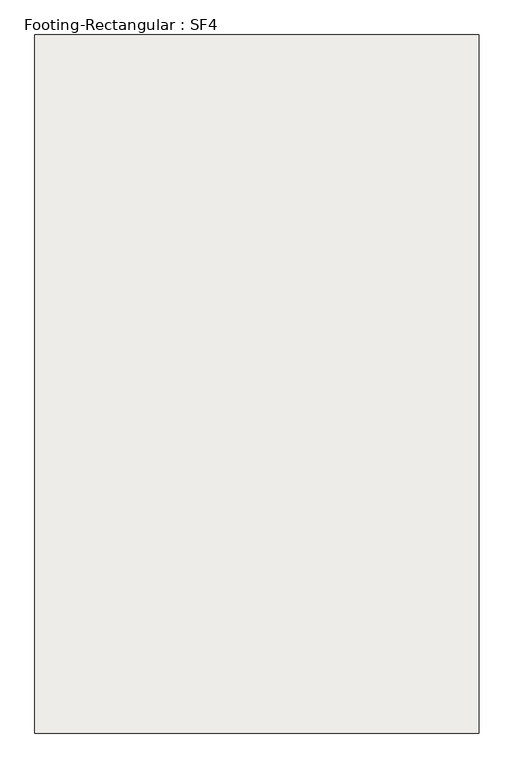
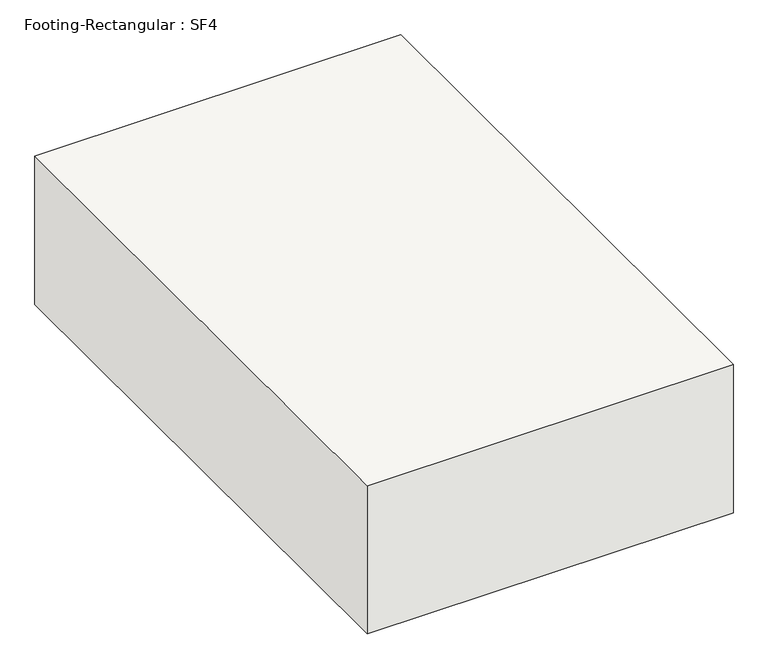
"""IFC4 building model written with IfcOpenShell, lengths in millimetres: slab geometry, Footing-Rectangular : SF4."""

from ifc_helpers import new_model, si_unit, frame, origin, place, context, project, spatial, polyline, outline, extrude, source, transform, mapped, element, save


def footing_rectangular_sf4_168fb1cd(model_context):
    return source(origin(), model_context, "Body", "SweptSolid", [
        extrude(outline(polyline([(533.4, 838.2), (533.4, -838.2), (-533.4, -838.2), (-533.4, 838.2), (533.4, 838.2)])), frame((0.0, 0.0, -457.2), z_axis=(0.0, 0.0, 1.0), x_axis=(1.0, 0.0, 0.0)), (0.0, 0.0, 1.0), 457.2),
    ])


if __name__ == "__main__":
    model = new_model("IFC4")
    model_context = context("Model", 3, world=origin())
    ifc_project = project(units=[si_unit("LENGTHUNIT", "METRE", prefix="MILLI")], contexts=[model_context])
    site = spatial("IfcSite", under=ifc_project)
    building = spatial("IfcBuilding", under=site)
    placement = place(None, origin())
    footing_rectangular_sf4_shape = footing_rectangular_sf4_168fb1cd(model_context)
    element("IfcSlab", 1, ObjectType="Footing-Rectangular : SF4", at=placement, inside=building, context=model_context, shape_type="MappedRepresentation", body=[
        mapped(footing_rectangular_sf4_shape, transform((0.0, 0.0, 0.0), x_axis=(1.0, 0.0, 0.0), y_axis=(0.0, 1.0, 0.0), z_axis=(0.0, 0.0, 1.0))),
    ])
    save(model, "model.ifc")

# Revit data of these elements
# Type "Footing-Rectangular : SF4"
#   Width = 1066.8 mm
#   Length = 1676.4 mm
#   Foundation Thickness = 457.2 mm
#   Structural Material [instance default] = Concrete - Cast-in-Place Concrete
#   Assembly Code = ""
# Element 1 (IfcSlab, "Footing-Rectangular : SF4")
#   Materials on its faces: "Concrete - Cast-in-Place Concrete"
# Materials
#   "Concrete - Cast-in-Place Concrete": class "Concrete", colour RGB 192 192 192, transparency 0, Cost = 0
